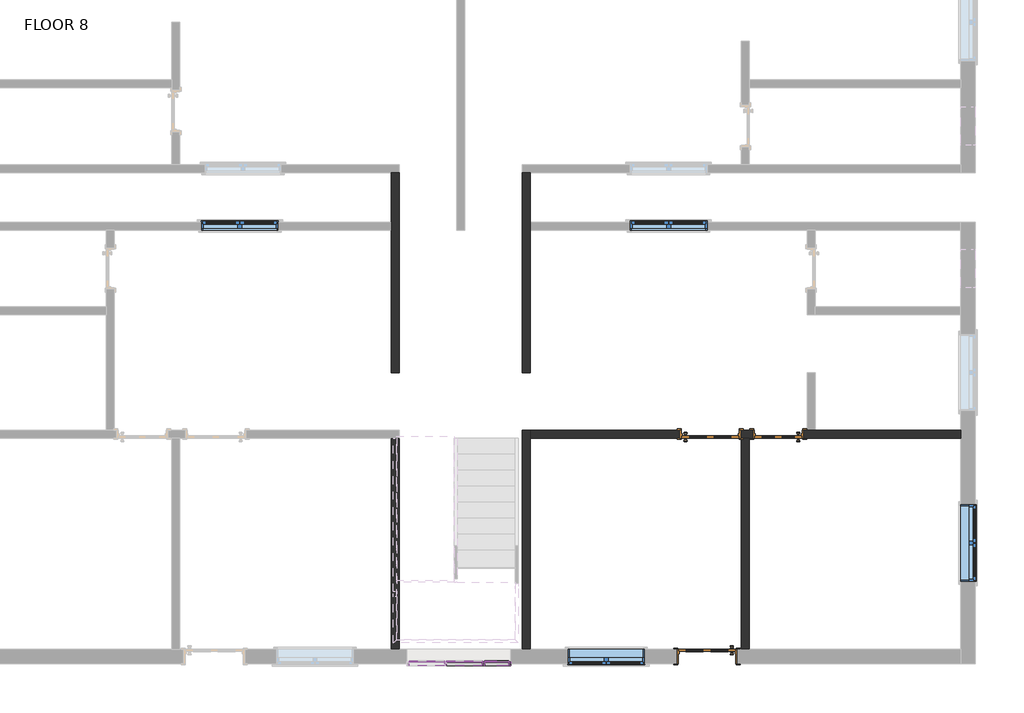
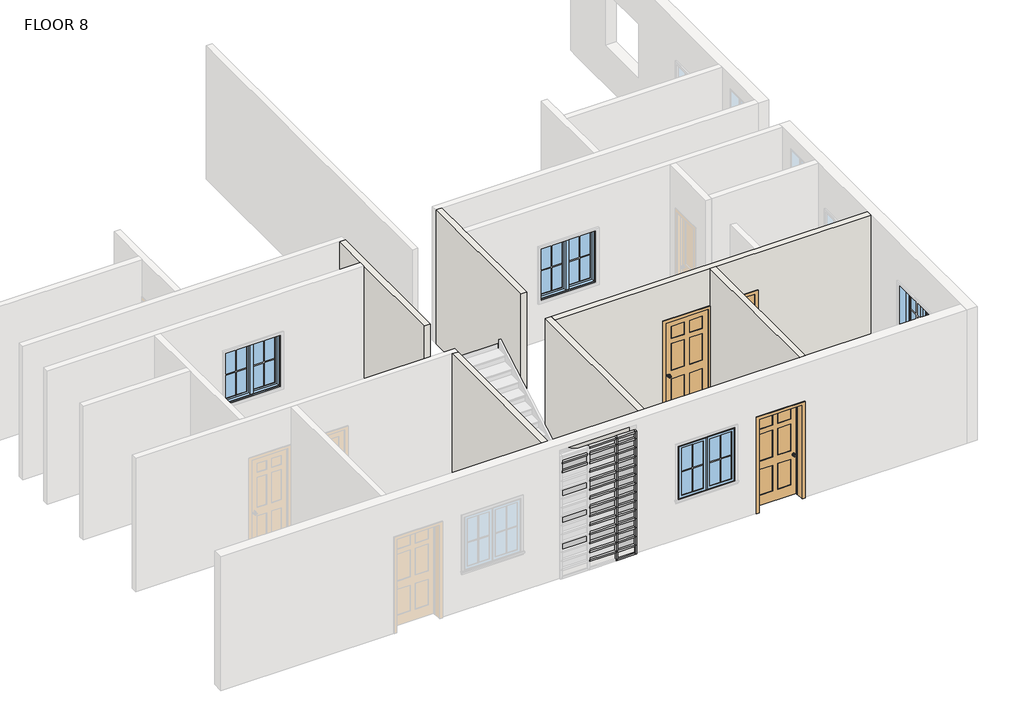
# One storey, part 2 of 4: 59 members, 22 plates, 6 walls, 4 windows, 3 doors.
"""IFC4 building model written with IfcOpenShell, lengths in millimetres."""

from ifc_helpers import new_model, si_unit, frame, origin, place, context, project, spatial, polyline, outline, extrude, faceted_brep, transform, mapped, element, save
from components import door_d66ee888, door_c610b25b, door_c5239341, member_56b223d9, member_a59c64b1, member_6a7c88b6, member_b8e7570c, member_a67f877f, member_ff422208, member_dc11c383, member_89338317, member_bd75388b, system_panel_glazed_b3845325, system_panel_glazed_23b8b45c, system_panel_glazed_a64eeae2, system_panel_glazed_c4340a26, system_panel_glazed_ac390e92, window_9200f5ac, window_c2c97eee

model = new_model("IFC4")

# Units and contexts
model_context = context("Model", 3, world=origin())
ifc_project = project(units=[si_unit("LENGTHUNIT", "METRE", prefix="MILLI")], contexts=[model_context])

# Site, building, storey
site = spatial("IfcSite", under=ifc_project)
building = spatial("IfcBuilding", under=site)
storey = spatial("IfcBuildingStorey", under=building, Name="FLOOR 8", Elevation=12744.7725604)

# Doors
placement = place(None, origin())
door_shape = door_d66ee888(model_context)
element("IfcDoor", 1, ObjectType="Door-Interior-Single-6_Panel-Wood : 30\" x 84\"", at=placement, inside=storey, context=model_context, shape_type="MappedRepresentation", body=[
    mapped(door_shape, transform((777.5862669, -4180.7343836, 12744.7725604), x_axis=(-1.0, 0.0, 0.0), y_axis=(0.0, -1.0, 0.0), z_axis=(0.0, 0.0, 1.0))),
])
door_2_shape = door_c610b25b(model_context)
element("IfcDoor", 2, ObjectType="Door-Interior-Single-6_Panel-Wood : 36\" x 84\"", at=placement, inside=storey, context=model_context, shape_type="MappedRepresentation", body=[
    mapped(door_2_shape, transform((-301.9137331, -4180.7343836, 12744.7725604), x_axis=(1.0, 0.0, 0.0), y_axis=(0.0, 1.0, 0.0), z_axis=(0.0, 0.0, 1.0))),
])
door_3_shape = door_c5239341(model_context)
element("IfcDoor", 3, ObjectType="Door-Interior-Single-6_Panel-Wood : 36\" x 84\"", at=placement, inside=storey, context=model_context, shape_type="MappedRepresentation", body=[
    mapped(door_3_shape, transform((-352.7137331, -7704.9843836, 12744.7725604), x_axis=(-1.0, 0.0, 0.0), y_axis=(0.0, -1.0, 0.0), z_axis=(0.0, 0.0, 1.0))),
])

# Members
member_shape = member_56b223d9(model_context)
element("IfcMember", 4, ObjectType="Rectangular Mullion : 1.5\" x 2.5\" rectangular", at=placement, inside=storey, context=model_context, shape_type="MappedRepresentation", body=[
    mapped(member_shape, transform((-3899.3003411, -7822.4593836, 12744.7725604), x_axis=(1.0, 0.0, 0.0), y_axis=(0.0, -1.0, 0.0), z_axis=(0.0, 0.0, -1.0))),
])
element("IfcMember", 5, ObjectType="Rectangular Mullion : 1.5\" x 2.5\" rectangular", at=placement, inside=storey, context=model_context, shape_type="MappedRepresentation", body=[
    mapped(member_shape, transform((-3899.3003411, -7822.4593836, 12947.9725604), x_axis=(1.0, 0.0, 0.0), y_axis=(0.0, -1.0, 0.0), z_axis=(0.0, 0.0, -1.0))),
])
element("IfcMember", 6, ObjectType="Rectangular Mullion : 1.5\" x 2.5\" rectangular", at=placement, inside=storey, context=model_context, shape_type="MappedRepresentation", body=[
    mapped(member_shape, transform((-3899.3003411, -7822.4593836, 13151.1725604), x_axis=(1.0, 0.0, 0.0), y_axis=(0.0, -1.0, 0.0), z_axis=(0.0, 0.0, -1.0))),
])
element("IfcMember", 7, ObjectType="Rectangular Mullion : 1.5\" x 2.5\" rectangular", at=placement, inside=storey, context=model_context, shape_type="MappedRepresentation", body=[
    mapped(member_shape, transform((-3899.3003411, -7822.4593836, 13354.3725604), x_axis=(1.0, 0.0, 0.0), y_axis=(0.0, -1.0, 0.0), z_axis=(0.0, 0.0, -1.0))),
])
element("IfcMember", 8, ObjectType="Rectangular Mullion : 1.5\" x 2.5\" rectangular", at=placement, inside=storey, context=model_context, shape_type="MappedRepresentation", body=[
    mapped(member_shape, transform((-3899.3003411, -7822.4593836, 13557.5725604), x_axis=(1.0, 0.0, 0.0), y_axis=(0.0, -1.0, 0.0), z_axis=(0.0, 0.0, -1.0))),
])
element("IfcMember", 9, ObjectType="Rectangular Mullion : 1.5\" x 2.5\" rectangular", at=placement, inside=storey, context=model_context, shape_type="MappedRepresentation", body=[
    mapped(member_shape, transform((-3899.3003411, -7822.4593836, 13760.7725604), x_axis=(1.0, 0.0, 0.0), y_axis=(0.0, -1.0, 0.0), z_axis=(0.0, 0.0, -1.0))),
])
element("IfcMember", 10, ObjectType="Rectangular Mullion : 1.5\" x 2.5\" rectangular", at=placement, inside=storey, context=model_context, shape_type="MappedRepresentation", body=[
    mapped(member_shape, transform((-3899.3003411, -7822.4593836, 13963.9725604), x_axis=(1.0, 0.0, 0.0), y_axis=(0.0, -1.0, 0.0), z_axis=(0.0, 0.0, -1.0))),
])
element("IfcMember", 11, ObjectType="Rectangular Mullion : 1.5\" x 2.5\" rectangular", at=placement, inside=storey, context=model_context, shape_type="MappedRepresentation", body=[
    mapped(member_shape, transform((-3899.3003411, -7822.4593836, 14167.1725604), x_axis=(1.0, 0.0, 0.0), y_axis=(0.0, -1.0, 0.0), z_axis=(0.0, 0.0, -1.0))),
])
element("IfcMember", 12, ObjectType="Rectangular Mullion : 1.5\" x 2.5\" rectangular", at=placement, inside=storey, context=model_context, shape_type="MappedRepresentation", body=[
    mapped(member_shape, transform((-3899.3003411, -7822.4593836, 14370.3725604), x_axis=(1.0, 0.0, 0.0), y_axis=(0.0, -1.0, 0.0), z_axis=(0.0, 0.0, -1.0))),
])
element("IfcMember", 13, ObjectType="Rectangular Mullion : 1.5\" x 2.5\" rectangular", at=placement, inside=storey, context=model_context, shape_type="MappedRepresentation", body=[
    mapped(member_shape, transform((-3899.3003411, -7822.4593836, 14573.5725604), x_axis=(1.0, 0.0, 0.0), y_axis=(0.0, -1.0, 0.0), z_axis=(0.0, 0.0, -1.0))),
])
element("IfcMember", 14, ObjectType="Rectangular Mullion : 1.5\" x 2.5\" rectangular", at=placement, inside=storey, context=model_context, shape_type="MappedRepresentation", body=[
    mapped(member_shape, transform((-3899.3003411, -7822.4593836, 14776.7725604), x_axis=(1.0, 0.0, 0.0), y_axis=(0.0, -1.0, 0.0), z_axis=(0.0, 0.0, -1.0))),
])
element("IfcMember", 15, ObjectType="Rectangular Mullion : 1.5\" x 2.5\" rectangular", at=placement, inside=storey, context=model_context, shape_type="MappedRepresentation", body=[
    mapped(member_shape, transform((-3899.3003411, -7822.4593836, 14979.9725604), x_axis=(1.0, 0.0, 0.0), y_axis=(0.0, -1.0, 0.0), z_axis=(0.0, 0.0, -1.0))),
])
element("IfcMember", 16, ObjectType="Rectangular Mullion : 1.5\" x 2.5\" rectangular", at=placement, inside=storey, context=model_context, shape_type="MappedRepresentation", body=[
    mapped(member_shape, transform((-3899.3003411, -7822.4593836, 15183.1725604), x_axis=(1.0, 0.0, 0.0), y_axis=(0.0, -1.0, 0.0), z_axis=(0.0, 0.0, -1.0))),
])
member_2_shape = member_a59c64b1(model_context)
element("IfcMember", 17, ObjectType="Rectangular Mullion : 1.5\" x 2.5\" rectangular", at=placement, inside=storey, context=model_context, shape_type="MappedRepresentation", body=[
    mapped(member_2_shape, transform((-3899.3003411, -7822.4593836, 15386.3725604), x_axis=(1.0, 0.0, 0.0), y_axis=(0.0, -1.0, 0.0), z_axis=(0.0, 0.0, -1.0))),
])
member_3_shape = member_6a7c88b6(model_context)
element("IfcMember", 18, ObjectType="Rectangular Mullion : 1.5\" x 2.5\" rectangular", at=placement, inside=storey, context=model_context, shape_type="MappedRepresentation", body=[
    mapped(member_3_shape, transform((-4527.9503411, -7822.4593836, 15183.1725604), x_axis=(0.0, 0.0, 1.0), y_axis=(0.0, -1.0, 0.0), z_axis=(1.0, 0.0, 0.0))),
])
element("IfcMember", 19, ObjectType="Rectangular Mullion : 1.5\" x 2.5\" rectangular", at=placement, inside=storey, context=model_context, shape_type="MappedRepresentation", body=[
    mapped(member_3_shape, transform((-4527.9503411, -7822.4593836, 15386.3725604), x_axis=(0.0, 0.0, 1.0), y_axis=(0.0, -1.0, 0.0), z_axis=(1.0, 0.0, 0.0))),
])
member_4_shape = member_b8e7570c(model_context)
element("IfcMember", 20, ObjectType="Rectangular Mullion : 1.5\" x 2.5\" rectangular", at=placement, inside=storey, context=model_context, shape_type="MappedRepresentation", body=[
    mapped(member_4_shape, transform((-3918.3503411, -7822.4593836, 12947.9725604), x_axis=(0.0, 0.0, 1.0), y_axis=(0.0, -1.0, 0.0), z_axis=(1.0, 0.0, 0.0))),
])
element("IfcMember", 21, ObjectType="Rectangular Mullion : 1.5\" x 2.5\" rectangular", at=placement, inside=storey, context=model_context, shape_type="MappedRepresentation", body=[
    mapped(member_4_shape, transform((-3918.3503411, -7822.4593836, 13151.1725604), x_axis=(0.0, 0.0, 1.0), y_axis=(0.0, -1.0, 0.0), z_axis=(1.0, 0.0, 0.0))),
])
element("IfcMember", 22, ObjectType="Rectangular Mullion : 1.5\" x 2.5\" rectangular", at=placement, inside=storey, context=model_context, shape_type="MappedRepresentation", body=[
    mapped(member_4_shape, transform((-3918.3503411, -7822.4593836, 13354.3725604), x_axis=(0.0, 0.0, 1.0), y_axis=(0.0, -1.0, 0.0), z_axis=(1.0, 0.0, 0.0))),
])
element("IfcMember", 23, ObjectType="Rectangular Mullion : 1.5\" x 2.5\" rectangular", at=placement, inside=storey, context=model_context, shape_type="MappedRepresentation", body=[
    mapped(member_4_shape, transform((-3918.3503411, -7822.4593836, 13557.5725604), x_axis=(0.0, 0.0, 1.0), y_axis=(0.0, -1.0, 0.0), z_axis=(1.0, 0.0, 0.0))),
])
element("IfcMember", 24, ObjectType="Rectangular Mullion : 1.5\" x 2.5\" rectangular", at=placement, inside=storey, context=model_context, shape_type="MappedRepresentation", body=[
    mapped(member_4_shape, transform((-3918.3503411, -7822.4593836, 13760.7725604), x_axis=(0.0, 0.0, 1.0), y_axis=(0.0, -1.0, 0.0), z_axis=(1.0, 0.0, 0.0))),
])
element("IfcMember", 25, ObjectType="Rectangular Mullion : 1.5\" x 2.5\" rectangular", at=placement, inside=storey, context=model_context, shape_type="MappedRepresentation", body=[
    mapped(member_4_shape, transform((-3918.3503411, -7822.4593836, 13963.9725604), x_axis=(0.0, 0.0, 1.0), y_axis=(0.0, -1.0, 0.0), z_axis=(1.0, 0.0, 0.0))),
])
element("IfcMember", 26, ObjectType="Rectangular Mullion : 1.5\" x 2.5\" rectangular", at=placement, inside=storey, context=model_context, shape_type="MappedRepresentation", body=[
    mapped(member_4_shape, transform((-3918.3503411, -7822.4593836, 14167.1725604), x_axis=(0.0, 0.0, 1.0), y_axis=(0.0, -1.0, 0.0), z_axis=(1.0, 0.0, 0.0))),
])
element("IfcMember", 27, ObjectType="Rectangular Mullion : 1.5\" x 2.5\" rectangular", at=placement, inside=storey, context=model_context, shape_type="MappedRepresentation", body=[
    mapped(member_4_shape, transform((-3918.3503411, -7822.4593836, 14370.3725604), x_axis=(0.0, 0.0, 1.0), y_axis=(0.0, -1.0, 0.0), z_axis=(1.0, 0.0, 0.0))),
])
element("IfcMember", 28, ObjectType="Rectangular Mullion : 1.5\" x 2.5\" rectangular", at=placement, inside=storey, context=model_context, shape_type="MappedRepresentation", body=[
    mapped(member_4_shape, transform((-3918.3503411, -7822.4593836, 14573.5725604), x_axis=(0.0, 0.0, 1.0), y_axis=(0.0, -1.0, 0.0), z_axis=(1.0, 0.0, 0.0))),
])
element("IfcMember", 29, ObjectType="Rectangular Mullion : 1.5\" x 2.5\" rectangular", at=placement, inside=storey, context=model_context, shape_type="MappedRepresentation", body=[
    mapped(member_4_shape, transform((-3918.3503411, -7822.4593836, 14776.7725604), x_axis=(0.0, 0.0, 1.0), y_axis=(0.0, -1.0, 0.0), z_axis=(1.0, 0.0, 0.0))),
])
element("IfcMember", 30, ObjectType="Rectangular Mullion : 1.5\" x 2.5\" rectangular", at=placement, inside=storey, context=model_context, shape_type="MappedRepresentation", body=[
    mapped(member_4_shape, transform((-3918.3503411, -7822.4593836, 14979.9725604), x_axis=(0.0, 0.0, 1.0), y_axis=(0.0, -1.0, 0.0), z_axis=(1.0, 0.0, 0.0))),
])
element("IfcMember", 31, ObjectType="Rectangular Mullion : 1.5\" x 2.5\" rectangular", at=placement, inside=storey, context=model_context, shape_type="MappedRepresentation", body=[
    mapped(member_4_shape, transform((-3918.3503411, -7822.4593836, 15183.1725604), x_axis=(0.0, 0.0, 1.0), y_axis=(0.0, -1.0, 0.0), z_axis=(1.0, 0.0, 0.0))),
])
element("IfcMember", 32, ObjectType="Rectangular Mullion : 1.5\" x 2.5\" rectangular", at=placement, inside=storey, context=model_context, shape_type="MappedRepresentation", body=[
    mapped(member_4_shape, transform((-3918.3503411, -7822.4593836, 15386.3725604), x_axis=(0.0, 0.0, 1.0), y_axis=(0.0, -1.0, 0.0), z_axis=(1.0, 0.0, 0.0))),
])
member_5_shape = member_a67f877f(model_context)
element("IfcMember", 33, ObjectType="Rectangular Mullion : 1.5\" x 2.5\" rectangular", at=placement, inside=storey, context=model_context, shape_type="MappedRepresentation", body=[
    mapped(member_5_shape, transform((-3918.3503411, -7822.4593836, 15552.1551755), x_axis=(0.0, 0.0, 1.0), y_axis=(0.0, -1.0, 0.0), z_axis=(1.0, 0.0, 0.0))),
])
member_6_shape = member_ff422208(model_context)
element("IfcMember", 34, ObjectType="Rectangular Mullion : 1.5\" x 2.5\" rectangular", at=placement, inside=storey, context=model_context, shape_type="MappedRepresentation", body=[
    mapped(member_6_shape, transform((-3466.9970483, -7822.4593836, 12744.7725604), x_axis=(1.0, 0.0, 0.0), y_axis=(0.0, -1.0, 0.0), z_axis=(0.0, 0.0, -1.0))),
])
element("IfcMember", 35, ObjectType="Rectangular Mullion : 1.5\" x 2.5\" rectangular", at=placement, inside=storey, context=model_context, shape_type="MappedRepresentation", body=[
    mapped(member_6_shape, transform((-3466.9970483, -7822.4593836, 12947.9725604), x_axis=(1.0, 0.0, 0.0), y_axis=(0.0, -1.0, 0.0), z_axis=(0.0, 0.0, -1.0))),
])
element("IfcMember", 36, ObjectType="Rectangular Mullion : 1.5\" x 2.5\" rectangular", at=placement, inside=storey, context=model_context, shape_type="MappedRepresentation", body=[
    mapped(member_6_shape, transform((-3466.9970483, -7822.4593836, 13151.1725604), x_axis=(1.0, 0.0, 0.0), y_axis=(0.0, -1.0, 0.0), z_axis=(0.0, 0.0, -1.0))),
])
element("IfcMember", 37, ObjectType="Rectangular Mullion : 1.5\" x 2.5\" rectangular", at=placement, inside=storey, context=model_context, shape_type="MappedRepresentation", body=[
    mapped(member_6_shape, transform((-3466.9970483, -7822.4593836, 13354.3725604), x_axis=(1.0, 0.0, 0.0), y_axis=(0.0, -1.0, 0.0), z_axis=(0.0, 0.0, -1.0))),
])
element("IfcMember", 38, ObjectType="Rectangular Mullion : 1.5\" x 2.5\" rectangular", at=placement, inside=storey, context=model_context, shape_type="MappedRepresentation", body=[
    mapped(member_6_shape, transform((-3466.9970483, -7822.4593836, 13557.5725604), x_axis=(1.0, 0.0, 0.0), y_axis=(0.0, -1.0, 0.0), z_axis=(0.0, 0.0, -1.0))),
])
element("IfcMember", 39, ObjectType="Rectangular Mullion : 1.5\" x 2.5\" rectangular", at=placement, inside=storey, context=model_context, shape_type="MappedRepresentation", body=[
    mapped(member_6_shape, transform((-3466.9970483, -7822.4593836, 13760.7725604), x_axis=(1.0, 0.0, 0.0), y_axis=(0.0, -1.0, 0.0), z_axis=(0.0, 0.0, -1.0))),
])
element("IfcMember", 40, ObjectType="Rectangular Mullion : 1.5\" x 2.5\" rectangular", at=placement, inside=storey, context=model_context, shape_type="MappedRepresentation", body=[
    mapped(member_6_shape, transform((-3466.9970483, -7822.4593836, 13963.9725604), x_axis=(1.0, 0.0, 0.0), y_axis=(0.0, -1.0, 0.0), z_axis=(0.0, 0.0, -1.0))),
])
element("IfcMember", 41, ObjectType="Rectangular Mullion : 1.5\" x 2.5\" rectangular", at=placement, inside=storey, context=model_context, shape_type="MappedRepresentation", body=[
    mapped(member_6_shape, transform((-3466.9970483, -7822.4593836, 14167.1725604), x_axis=(1.0, 0.0, 0.0), y_axis=(0.0, -1.0, 0.0), z_axis=(0.0, 0.0, -1.0))),
])
element("IfcMember", 42, ObjectType="Rectangular Mullion : 1.5\" x 2.5\" rectangular", at=placement, inside=storey, context=model_context, shape_type="MappedRepresentation", body=[
    mapped(member_6_shape, transform((-3466.9970483, -7822.4593836, 14370.3725604), x_axis=(1.0, 0.0, 0.0), y_axis=(0.0, -1.0, 0.0), z_axis=(0.0, 0.0, -1.0))),
])
element("IfcMember", 43, ObjectType="Rectangular Mullion : 1.5\" x 2.5\" rectangular", at=placement, inside=storey, context=model_context, shape_type="MappedRepresentation", body=[
    mapped(member_6_shape, transform((-3466.9970483, -7822.4593836, 14573.5725604), x_axis=(1.0, 0.0, 0.0), y_axis=(0.0, -1.0, 0.0), z_axis=(0.0, 0.0, -1.0))),
])
element("IfcMember", 44, ObjectType="Rectangular Mullion : 1.5\" x 2.5\" rectangular", at=placement, inside=storey, context=model_context, shape_type="MappedRepresentation", body=[
    mapped(member_6_shape, transform((-3466.9970483, -7822.4593836, 14776.7725604), x_axis=(1.0, 0.0, 0.0), y_axis=(0.0, -1.0, 0.0), z_axis=(0.0, 0.0, -1.0))),
])
element("IfcMember", 45, ObjectType="Rectangular Mullion : 1.5\" x 2.5\" rectangular", at=placement, inside=storey, context=model_context, shape_type="MappedRepresentation", body=[
    mapped(member_6_shape, transform((-3466.9970483, -7822.4593836, 14979.9725604), x_axis=(1.0, 0.0, 0.0), y_axis=(0.0, -1.0, 0.0), z_axis=(0.0, 0.0, -1.0))),
])
element("IfcMember", 46, ObjectType="Rectangular Mullion : 1.5\" x 2.5\" rectangular", at=placement, inside=storey, context=model_context, shape_type="MappedRepresentation", body=[
    mapped(member_6_shape, transform((-3466.9970483, -7822.4593836, 15183.1725604), x_axis=(1.0, 0.0, 0.0), y_axis=(0.0, -1.0, 0.0), z_axis=(0.0, 0.0, -1.0))),
])
member_7_shape = member_dc11c383(model_context)
element("IfcMember", 47, ObjectType="Rectangular Mullion : 1.5\" x 2.5\" rectangular", at=placement, inside=storey, context=model_context, shape_type="MappedRepresentation", body=[
    mapped(member_7_shape, transform((-3466.9970483, -7822.4593836, 15386.3725604), x_axis=(1.0, 0.0, 0.0), y_axis=(0.0, -1.0, 0.0), z_axis=(0.0, 0.0, -1.0))),
])
member_8_shape = member_89338317(model_context)
element("IfcMember", 48, ObjectType="Rectangular Mullion : 1.5\" x 2.5\" rectangular", at=placement, inside=storey, context=model_context, shape_type="MappedRepresentation", body=[
    mapped(member_8_shape, transform((-3505.0970483, -7822.4593836, 15552.1551755), x_axis=(0.0, 0.0, 1.0), y_axis=(0.0, -1.0, 0.0), z_axis=(1.0, 0.0, 0.0))),
])
element("IfcMember", 49, ObjectType="Rectangular Mullion : 1.5\" x 2.5\" rectangular", at=placement, inside=storey, context=model_context, shape_type="MappedRepresentation", body=[
    mapped(member_8_shape, transform((-3880.2503411, -7822.4593836, 12744.7725604), x_axis=(0.0, 0.0, -1.0), y_axis=(0.0, -1.0, 0.0), z_axis=(-1.0, 0.0, 0.0))),
])
member_9_shape = member_bd75388b(model_context)
element("IfcMember", 50, ObjectType="Rectangular Mullion : 1.5\" x 2.5\" rectangular", at=placement, inside=storey, context=model_context, shape_type="MappedRepresentation", body=[
    mapped(member_9_shape, transform((-3505.0970483, -7822.4593836, 12947.9725604), x_axis=(0.0, 0.0, 1.0), y_axis=(0.0, -1.0, 0.0), z_axis=(1.0, 0.0, 0.0))),
])
element("IfcMember", 51, ObjectType="Rectangular Mullion : 1.5\" x 2.5\" rectangular", at=placement, inside=storey, context=model_context, shape_type="MappedRepresentation", body=[
    mapped(member_9_shape, transform((-3505.0970483, -7822.4593836, 13151.1725604), x_axis=(0.0, 0.0, 1.0), y_axis=(0.0, -1.0, 0.0), z_axis=(1.0, 0.0, 0.0))),
])
element("IfcMember", 52, ObjectType="Rectangular Mullion : 1.5\" x 2.5\" rectangular", at=placement, inside=storey, context=model_context, shape_type="MappedRepresentation", body=[
    mapped(member_9_shape, transform((-3505.0970483, -7822.4593836, 13354.3725604), x_axis=(0.0, 0.0, 1.0), y_axis=(0.0, -1.0, 0.0), z_axis=(1.0, 0.0, 0.0))),
])
element("IfcMember", 53, ObjectType="Rectangular Mullion : 1.5\" x 2.5\" rectangular", at=placement, inside=storey, context=model_context, shape_type="MappedRepresentation", body=[
    mapped(member_9_shape, transform((-3505.0970483, -7822.4593836, 13557.5725604), x_axis=(0.0, 0.0, 1.0), y_axis=(0.0, -1.0, 0.0), z_axis=(1.0, 0.0, 0.0))),
])
element("IfcMember", 54, ObjectType="Rectangular Mullion : 1.5\" x 2.5\" rectangular", at=placement, inside=storey, context=model_context, shape_type="MappedRepresentation", body=[
    mapped(member_9_shape, transform((-3505.0970483, -7822.4593836, 13760.7725604), x_axis=(0.0, 0.0, 1.0), y_axis=(0.0, -1.0, 0.0), z_axis=(1.0, 0.0, 0.0))),
])
element("IfcMember", 55, ObjectType="Rectangular Mullion : 1.5\" x 2.5\" rectangular", at=placement, inside=storey, context=model_context, shape_type="MappedRepresentation", body=[
    mapped(member_9_shape, transform((-3505.0970483, -7822.4593836, 13963.9725604), x_axis=(0.0, 0.0, 1.0), y_axis=(0.0, -1.0, 0.0), z_axis=(1.0, 0.0, 0.0))),
])
element("IfcMember", 56, ObjectType="Rectangular Mullion : 1.5\" x 2.5\" rectangular", at=placement, inside=storey, context=model_context, shape_type="MappedRepresentation", body=[
    mapped(member_9_shape, transform((-3505.0970483, -7822.4593836, 14167.1725604), x_axis=(0.0, 0.0, 1.0), y_axis=(0.0, -1.0, 0.0), z_axis=(1.0, 0.0, 0.0))),
])
element("IfcMember", 57, ObjectType="Rectangular Mullion : 1.5\" x 2.5\" rectangular", at=placement, inside=storey, context=model_context, shape_type="MappedRepresentation", body=[
    mapped(member_9_shape, transform((-3505.0970483, -7822.4593836, 14370.3725604), x_axis=(0.0, 0.0, 1.0), y_axis=(0.0, -1.0, 0.0), z_axis=(1.0, 0.0, 0.0))),
])
element("IfcMember", 58, ObjectType="Rectangular Mullion : 1.5\" x 2.5\" rectangular", at=placement, inside=storey, context=model_context, shape_type="MappedRepresentation", body=[
    mapped(member_9_shape, transform((-3505.0970483, -7822.4593836, 14573.5725604), x_axis=(0.0, 0.0, 1.0), y_axis=(0.0, -1.0, 0.0), z_axis=(1.0, 0.0, 0.0))),
])
element("IfcMember", 59, ObjectType="Rectangular Mullion : 1.5\" x 2.5\" rectangular", at=placement, inside=storey, context=model_context, shape_type="MappedRepresentation", body=[
    mapped(member_9_shape, transform((-3505.0970483, -7822.4593836, 14776.7725604), x_axis=(0.0, 0.0, 1.0), y_axis=(0.0, -1.0, 0.0), z_axis=(1.0, 0.0, 0.0))),
])
element("IfcMember", 60, ObjectType="Rectangular Mullion : 1.5\" x 2.5\" rectangular", at=placement, inside=storey, context=model_context, shape_type="MappedRepresentation", body=[
    mapped(member_9_shape, transform((-3505.0970483, -7822.4593836, 14979.9725604), x_axis=(0.0, 0.0, 1.0), y_axis=(0.0, -1.0, 0.0), z_axis=(1.0, 0.0, 0.0))),
])
element("IfcMember", 61, ObjectType="Rectangular Mullion : 1.5\" x 2.5\" rectangular", at=placement, inside=storey, context=model_context, shape_type="MappedRepresentation", body=[
    mapped(member_9_shape, transform((-3505.0970483, -7822.4593836, 15183.1725604), x_axis=(0.0, 0.0, 1.0), y_axis=(0.0, -1.0, 0.0), z_axis=(1.0, 0.0, 0.0))),
])
element("IfcMember", 62, ObjectType="Rectangular Mullion : 1.5\" x 2.5\" rectangular", at=placement, inside=storey, context=model_context, shape_type="MappedRepresentation", body=[
    mapped(member_9_shape, transform((-3505.0970483, -7822.4593836, 15386.3725604), x_axis=(0.0, 0.0, 1.0), y_axis=(0.0, -1.0, 0.0), z_axis=(1.0, 0.0, 0.0))),
])

# Plates
system_panel_glazed_shape = system_panel_glazed_b3845325(model_context)
element("IfcPlate", 63, ObjectType="System Panel : Glazed", at=placement, inside=storey, context=model_context, shape_type="MappedRepresentation", body=[
    mapped(system_panel_glazed_shape, transform((-4804.1753412, -7822.4593836, 13373.4225604), x_axis=(1.0, 0.0, 0.0), y_axis=(0.0, 1.0, 0.0), z_axis=(0.0, 0.0, 1.0))),
])
element("IfcPlate", 64, ObjectType="System Panel : Glazed", at=placement, inside=storey, context=model_context, shape_type="MappedRepresentation", body=[
    mapped(system_panel_glazed_shape, transform((-4804.1753412, -7822.4593836, 13983.0225604), x_axis=(1.0, 0.0, 0.0), y_axis=(0.0, 1.0, 0.0), z_axis=(0.0, 0.0, 1.0))),
])
element("IfcPlate", 65, ObjectType="System Panel : Glazed", at=placement, inside=storey, context=model_context, shape_type="MappedRepresentation", body=[
    mapped(system_panel_glazed_shape, transform((-4804.1753412, -7822.4593836, 14592.6225604), x_axis=(1.0, 0.0, 0.0), y_axis=(0.0, 1.0, 0.0), z_axis=(0.0, 0.0, 1.0))),
])
element("IfcPlate", 66, ObjectType="System Panel : Glazed", at=placement, inside=storey, context=model_context, shape_type="MappedRepresentation", body=[
    mapped(system_panel_glazed_shape, transform((-4804.1753412, -7822.4593836, 15202.2225604), x_axis=(1.0, 0.0, 0.0), y_axis=(0.0, 1.0, 0.0), z_axis=(0.0, 0.0, 1.0))),
])
system_panel_glazed_2_shape = system_panel_glazed_23b8b45c(model_context)
element("IfcPlate", 67, ObjectType="System Panel : Glazed", at=placement, inside=storey, context=model_context, shape_type="MappedRepresentation", body=[
    mapped(system_panel_glazed_2_shape, transform((-4204.1003411, -7822.4593836, 13373.4225604), x_axis=(1.0, 0.0, 0.0), y_axis=(0.0, 1.0, 0.0), z_axis=(0.0, 0.0, 1.0))),
])
element("IfcPlate", 68, ObjectType="System Panel : Glazed", at=placement, inside=storey, context=model_context, shape_type="MappedRepresentation", body=[
    mapped(system_panel_glazed_2_shape, transform((-4204.1003411, -7822.4593836, 13983.0225604), x_axis=(1.0, 0.0, 0.0), y_axis=(0.0, 1.0, 0.0), z_axis=(0.0, 0.0, 1.0))),
])
element("IfcPlate", 69, ObjectType="System Panel : Glazed", at=placement, inside=storey, context=model_context, shape_type="MappedRepresentation", body=[
    mapped(system_panel_glazed_2_shape, transform((-4204.1003411, -7822.4593836, 14592.6225604), x_axis=(1.0, 0.0, 0.0), y_axis=(0.0, 1.0, 0.0), z_axis=(0.0, 0.0, 1.0))),
])
element("IfcPlate", 70, ObjectType="System Panel : Glazed", at=placement, inside=storey, context=model_context, shape_type="MappedRepresentation", body=[
    mapped(system_panel_glazed_2_shape, transform((-4204.1003411, -7822.4593836, 15202.2225604), x_axis=(1.0, 0.0, 0.0), y_axis=(0.0, 1.0, 0.0), z_axis=(0.0, 0.0, 1.0))),
])
system_panel_glazed_3_shape = system_panel_glazed_a64eeae2(model_context)
element("IfcPlate", 71, ObjectType="System Panel : Glazed", at=placement, inside=storey, context=model_context, shape_type="MappedRepresentation", body=[
    mapped(system_panel_glazed_3_shape, transform((-3692.6736947, -7822.4593836, 12782.8725604), x_axis=(1.0, 0.0, 0.0), y_axis=(0.0, 1.0, 0.0), z_axis=(0.0, 0.0, 1.0))),
])
system_panel_glazed_4_shape = system_panel_glazed_c4340a26(model_context)
element("IfcPlate", 72, ObjectType="System Panel : Glazed", at=placement, inside=storey, context=model_context, shape_type="MappedRepresentation", body=[
    mapped(system_panel_glazed_4_shape, transform((-3692.6736947, -7822.4593836, 12967.0225604), x_axis=(1.0, 0.0, 0.0), y_axis=(0.0, 1.0, 0.0), z_axis=(0.0, 0.0, 1.0))),
])
element("IfcPlate", 73, ObjectType="System Panel : Glazed", at=placement, inside=storey, context=model_context, shape_type="MappedRepresentation", body=[
    mapped(system_panel_glazed_4_shape, transform((-3692.6736947, -7822.4593836, 13170.2225604), x_axis=(1.0, 0.0, 0.0), y_axis=(0.0, 1.0, 0.0), z_axis=(0.0, 0.0, 1.0))),
])
element("IfcPlate", 74, ObjectType="System Panel : Glazed", at=placement, inside=storey, context=model_context, shape_type="MappedRepresentation", body=[
    mapped(system_panel_glazed_4_shape, transform((-3692.6736947, -7822.4593836, 13576.6225604), x_axis=(1.0, 0.0, 0.0), y_axis=(0.0, 1.0, 0.0), z_axis=(0.0, 0.0, 1.0))),
])
element("IfcPlate", 75, ObjectType="System Panel : Glazed", at=placement, inside=storey, context=model_context, shape_type="MappedRepresentation", body=[
    mapped(system_panel_glazed_4_shape, transform((-3692.6736947, -7822.4593836, 13779.8225604), x_axis=(1.0, 0.0, 0.0), y_axis=(0.0, 1.0, 0.0), z_axis=(0.0, 0.0, 1.0))),
])
element("IfcPlate", 76, ObjectType="System Panel : Glazed", at=placement, inside=storey, context=model_context, shape_type="MappedRepresentation", body=[
    mapped(system_panel_glazed_4_shape, transform((-3692.6736947, -7822.4593836, 14186.2225604), x_axis=(1.0, 0.0, 0.0), y_axis=(0.0, 1.0, 0.0), z_axis=(0.0, 0.0, 1.0))),
])
element("IfcPlate", 77, ObjectType="System Panel : Glazed", at=placement, inside=storey, context=model_context, shape_type="MappedRepresentation", body=[
    mapped(system_panel_glazed_4_shape, transform((-3692.6736947, -7822.4593836, 14389.4225604), x_axis=(1.0, 0.0, 0.0), y_axis=(0.0, 1.0, 0.0), z_axis=(0.0, 0.0, 1.0))),
])
element("IfcPlate", 78, ObjectType="System Panel : Glazed", at=placement, inside=storey, context=model_context, shape_type="MappedRepresentation", body=[
    mapped(system_panel_glazed_4_shape, transform((-3692.6736947, -7822.4593836, 14795.8225604), x_axis=(1.0, 0.0, 0.0), y_axis=(0.0, 1.0, 0.0), z_axis=(0.0, 0.0, 1.0))),
])
element("IfcPlate", 79, ObjectType="System Panel : Glazed", at=placement, inside=storey, context=model_context, shape_type="MappedRepresentation", body=[
    mapped(system_panel_glazed_4_shape, transform((-3692.6736947, -7822.4593836, 14999.0225604), x_axis=(1.0, 0.0, 0.0), y_axis=(0.0, 1.0, 0.0), z_axis=(0.0, 0.0, 1.0))),
])
element("IfcPlate", 80, ObjectType="System Panel : Glazed", at=placement, inside=storey, context=model_context, shape_type="MappedRepresentation", body=[
    mapped(system_panel_glazed_4_shape, transform((-3692.6736947, -7822.4593836, 13373.4225604), x_axis=(1.0, 0.0, 0.0), y_axis=(0.0, 1.0, 0.0), z_axis=(0.0, 0.0, 1.0))),
])
element("IfcPlate", 81, ObjectType="System Panel : Glazed", at=placement, inside=storey, context=model_context, shape_type="MappedRepresentation", body=[
    mapped(system_panel_glazed_4_shape, transform((-3692.6736947, -7822.4593836, 13983.0225604), x_axis=(1.0, 0.0, 0.0), y_axis=(0.0, 1.0, 0.0), z_axis=(0.0, 0.0, 1.0))),
])
element("IfcPlate", 82, ObjectType="System Panel : Glazed", at=placement, inside=storey, context=model_context, shape_type="MappedRepresentation", body=[
    mapped(system_panel_glazed_4_shape, transform((-3692.6736947, -7822.4593836, 14592.6225604), x_axis=(1.0, 0.0, 0.0), y_axis=(0.0, 1.0, 0.0), z_axis=(0.0, 0.0, 1.0))),
])
element("IfcPlate", 83, ObjectType="System Panel : Glazed", at=placement, inside=storey, context=model_context, shape_type="MappedRepresentation", body=[
    mapped(system_panel_glazed_4_shape, transform((-3692.6736947, -7822.4593836, 15202.2225604), x_axis=(1.0, 0.0, 0.0), y_axis=(0.0, 1.0, 0.0), z_axis=(0.0, 0.0, 1.0))),
])
system_panel_glazed_5_shape = system_panel_glazed_ac390e92(model_context)
element("IfcPlate", 84, ObjectType="System Panel : Glazed", at=placement, inside=storey, context=model_context, shape_type="MappedRepresentation", body=[
    mapped(system_panel_glazed_5_shape, transform((-3692.6736947, -7822.4593836, 15405.4225604), x_axis=(1.0, 0.0, 0.0), y_axis=(0.0, 1.0, 0.0), z_axis=(0.0, 0.0, 1.0))),
])

# Walls
element("IfcWall", 85, ObjectType="Inner Wall 5\"", at=placement, inside=storey, context=model_context, shape_type="Brep", body=[
    faceted_brep([(-5369.2137331, -24.6593836, 12744.7725604), (-5369.2137331, -812.0593836, 12744.7725604), (-5369.2137331, -939.0593836, 12744.7725604), (-5369.2137331, -3199.6593836, 12744.7725604), (-5369.2137331, -3199.6593836, 15792.7725604), (-5369.2137331, -939.0593836, 15792.7725604), (-5369.2137331, -812.0593836, 15792.7725604), (-5369.2137331, -24.6593836, 15792.7725604), (-5242.2137331, -24.6593836, 12744.7725604), (-5242.2137331, -24.6593836, 15792.7725604), (-5242.2137331, -3199.6593836, 15792.7725604), (-5242.2137331, -3199.6593836, 12744.7725604)], [[[0, 1, 2, 3, 4, 5, 6, 7]], [[8, 9, 10, 11]], [[3, 2, 1, 0, 8, 11]], [[4, 3, 11, 10]], [[7, 6, 5, 4, 10, 9]], [[0, 7, 9, 8]]]),
])
element("IfcWall", 86, ObjectType="Inner Wall 5\"", at=placement, inside=storey, context=model_context, shape_type="Brep", body=[
    faceted_brep([(-3286.4137331, -24.6593836, 12744.7725604), (-3286.4137331, -3199.6593836, 12744.7725604), (-3286.4137331, -3199.6593836, 15792.7725604), (-3286.4137331, -24.6593836, 15792.7725604), (-3159.4137331, -24.6593836, 12744.7725604), (-3159.4137331, -24.6593836, 15792.7725604), (-3159.4137331, -812.0593836, 15792.7725604), (-3159.4137331, -939.0593836, 15792.7725604), (-3159.4137331, -3199.6593836, 15792.7725604), (-3159.4137331, -3199.6593836, 12744.7725604), (-3159.4137331, -939.0593836, 12744.7725604), (-3159.4137331, -812.0593836, 12744.7725604)], [[[0, 1, 2, 3]], [[4, 5, 6, 7, 8, 9, 10, 11]], [[1, 0, 4, 11, 10, 9]], [[2, 1, 9, 8]], [[3, 2, 8, 7, 6, 5]], [[0, 3, 5, 4]]]),
])
element("IfcWall", 87, ObjectType="Inner Wall 5\"", at=placement, inside=storey, context=model_context, shape_type="SweptSolid", body=[
    extrude(outline(polyline([(-5242.2137331, -4241.0593836), (-5242.2137331, -7593.8593836), (-5369.2137331, -7593.8593836), (-5369.2137331, -4241.0593836), (-5242.2137331, -4241.0593836)])), frame((0.0, 0.0, 12744.7725604), z_axis=(0.0, 0.0, 1.0), x_axis=(1.0, 0.0, 0.0)), (0.0, 0.0, 1.0), 3048.0),
])
element("IfcWall", 88, ObjectType="Inner Wall 5\"", at=placement, inside=storey, context=model_context, shape_type="Brep", body=[
    faceted_brep([(-3159.4137331, -7593.8593836, 12744.7725604), (-3159.4137331, -4241.0593836, 12744.7725604), (-3159.4137331, -4114.0593836, 12744.7725604), (-3159.4137331, -4114.0593836, 15792.7725604), (-3159.4137331, -4241.0593836, 15792.7725604), (-3159.4137331, -7593.8593836, 15792.7725604), (-3286.4137331, -7593.8593836, 12744.7725604), (-3286.4137331, -7593.8593836, 15792.7725604), (-3286.4137331, -4114.0593836, 15792.7725604), (-3286.4137331, -4114.0593836, 12744.7725604)], [[[0, 1, 2, 3, 4, 5]], [[6, 7, 8, 9]], [[2, 1, 0, 6, 9]], [[5, 4, 3, 8, 7]], [[0, 5, 7, 6]], [[3, 2, 9, 8]]]),
])
element("IfcWall", 89, ObjectType="Inner Wall 5\"", at=placement, inside=storey, context=model_context, shape_type="Brep", body=[
    faceted_brep([(3673.1862669, -4241.0593836, 15792.7725604), (320.3862669, -4241.0593836, 15792.7725604), (193.3862669, -4241.0593836, 15792.7725604), (-3159.4137331, -4241.0593836, 15792.7725604), (-3159.4137331, -4241.0593836, 12744.7725604), (-784.5137331, -4241.0593836, 12744.7725604), (-784.5137331, -4241.0593836, 14903.7725604), (180.6862669, -4241.0593836, 14903.7725604), (180.6862669, -4241.0593836, 12744.7725604), (193.3862669, -4241.0593836, 12744.7725604), (320.3862669, -4241.0593836, 12744.7725604), (371.1862669, -4241.0593836, 12744.7725604), (371.1862669, -4241.0593836, 14903.7725604), (1183.9862669, -4241.0593836, 14903.7725604), (1183.9862669, -4241.0593836, 12744.7725604), (3673.1862669, -4241.0593836, 12744.7725604), (-3159.4137331, -4114.0593836, 15792.7725604), (1234.7862669, -4114.0593836, 15792.7725604), (1361.7862669, -4114.0593836, 15792.7725604), (3673.1862669, -4114.0593836, 15792.7725604), (3673.1862669, -4114.0593836, 12744.7725604), (1361.7862669, -4114.0593836, 12744.7725604), (1234.7862669, -4114.0593836, 12744.7725604), (1183.9862669, -4114.0593836, 12744.7725604), (1183.9862669, -4114.0593836, 14903.7725604), (371.1862669, -4114.0593836, 14903.7725604), (371.1862669, -4114.0593836, 12744.7725604), (180.6862669, -4114.0593836, 12744.7725604), (180.6862669, -4114.0593836, 14903.7725604), (-784.5137331, -4114.0593836, 14903.7725604), (-784.5137331, -4114.0593836, 12744.7725604), (-3159.4137331, -4114.0593836, 12744.7725604)], [[[0, 1, 2, 3, 4, 5, 6, 7, 8, 9, 10, 11, 12, 13, 14, 15]], [[16, 17, 18, 19, 20, 21, 22, 23, 24, 25, 26, 27, 28, 29, 30, 31]], [[4, 31, 30, 5]], [[20, 15, 14, 23, 22, 21]], [[8, 27, 26, 11, 10, 9]], [[3, 2, 1, 0, 19, 18, 17, 16]], [[4, 3, 16, 31]], [[0, 15, 20, 19]], [[7, 28, 27, 8]], [[28, 7, 6, 29]], [[29, 6, 5, 30]], [[25, 12, 11, 26]], [[12, 25, 24, 13]], [[13, 24, 23, 14]]]),
])
element("IfcWall", 90, ObjectType="Inner Wall 5\"", at=placement, inside=storey, context=model_context, shape_type="SweptSolid", body=[
    extrude(outline(polyline([(320.3862669, -4241.0593836), (320.3862669, -7593.8593836), (193.3862669, -7593.8593836), (193.3862669, -4241.0593836), (320.3862669, -4241.0593836)])), frame((0.0, 0.0, 12744.7725604), z_axis=(0.0, 0.0, 1.0), x_axis=(1.0, 0.0, 0.0)), (0.0, 0.0, 1.0), 3048.0),
])

# Windows
window_shape = window_9200f5ac(model_context)
element("IfcWindow", 91, ObjectType="Window-Casement-Double : 48\" x 48\"", at=placement, inside=storey, context=model_context, shape_type="MappedRepresentation", body=[
    mapped(window_shape, transform((3787.4862669, -5904.7593836, 12744.7725604), x_axis=(0.0, -1.0, 0.0), y_axis=(1.0, 0.0, 0.0), z_axis=(0.0, 0.0, 1.0))),
])
element("IfcWindow", 92, ObjectType="Window-Casement-Double : 48\" x 48\"", at=placement, inside=storey, context=model_context, shape_type="MappedRepresentation", body=[
    mapped(window_shape, transform((-1952.9137331, -7708.1593836, 12744.7725604), x_axis=(-1.0, 0.0, 0.0), y_axis=(0.0, -1.0, 0.0), z_axis=(0.0, 0.0, 1.0))),
])
window_2_shape = window_c2c97eee(model_context)
element("IfcWindow", 93, ObjectType="Window-Casement-Double : 48\" x 48\"", at=placement, inside=storey, context=model_context, shape_type="MappedRepresentation", body=[
    mapped(window_2_shape, transform((-7769.5137331, -875.5593836, 12744.7725604), x_axis=(1.0, 0.0, 0.0), y_axis=(0.0, 1.0, 0.0), z_axis=(0.0, 0.0, 1.0))),
])
element("IfcWindow", 94, ObjectType="Window-Casement-Double : 48\" x 48\"", at=placement, inside=storey, context=model_context, shape_type="MappedRepresentation", body=[
    mapped(window_2_shape, transform((-962.3137331, -875.5593836, 12744.7725604), x_axis=(1.0, 0.0, 0.0), y_axis=(0.0, 1.0, 0.0), z_axis=(0.0, 0.0, 1.0))),
])

save(model, "model.ifc")

# Revit data of these elements
# Type "Door-Interior-Single-6_Panel-Wood : 30\" x 84\""
#   Type Mark = "9"
#   Assembly Code = "C1020300"
#   Analytic Construction = "Wooden"
#   Top Rail = 0' - 4 11/16"
#   Top Panel = 0' - 8"
#   Thickness = 0' - 1 3/8"
#   Thermal Resistance (R) = 2.5876 (h·ft²·°F)/BTU
#   Swing Angle [instance default] = 90.00°
#   Stiles = 0' - 4 3/4"
#   Rough Width = 2' - 8"
#   Rough Height = 7' - 1"
#   Mullion = 0' - 4 1/2"
#   Lock Rail = 0' - 7 1/2"
#   Intermediate Rail = 0' - 4 1/2"
#   Height = 7' - 0"
#   Width = 2' - 6"
#   Heat Transfer Coefficient (U) = 0.3865 BTU/(h·ft²·°F)
#   Bottom Rail = 0' - 9 1/8"
#   Trim Material = Cherry
#   Panel Material = Cherry
#   Frame Material = Cherry
#   Door Handle Material = Aluminum
#   Visual Light Transmittance = 0
#   Solar Heat Gain Coefficient = 0
#   Wall Closure = (empty or 0)
#   Function = (empty or 0)
# Type "Door-Interior-Single-6_Panel-Wood : 36\" x 84\""
#   Type Mark = "8"
#   Assembly Code = "C1020300"
#   Analytic Construction = "Wooden"
#   Top Rail = 0' - 4 11/16"
#   Top Panel = 0' - 11"
#   Thickness = 0' - 1 3/8"
#   Thermal Resistance (R) = 2.5876 (h·ft²·°F)/BTU
#   Swing Angle [instance default] = 90.00°
#   Stiles = 0' - 4 3/4"
#   Rough Width = 3' - 2"
#   Rough Height = 7' - 1"
#   Mullion = 0' - 4 1/2"
#   Lock Rail = 0' - 7 1/2"
#   Intermediate Rail = 0' - 4 1/2"
#   Height = 7' - 0"
#   Width = 3' - 0"
#   Heat Transfer Coefficient (U) = 0.3865 BTU/(h·ft²·°F)
#   Bottom Rail = 0' - 9 1/8"
#   Trim Material = Cherry
#   Panel Material = Cherry
#   Frame Material = Cherry
#   Door Handle Material = Aluminum
#   Visual Light Transmittance = 0
#   Solar Heat Gain Coefficient = 0
#   Wall Closure = (empty or 0)
#   Function = (empty or 0)
# Type "Rectangular Mullion : 1.5\" x 2.5\" rectangular"
#   built-in parameter 1007304 = 0.208333 (stored number, unit not read)
#   built-in parameter 1007301 = 0.0625 (stored number, unit not read)
#   built-in parameter 1007300 = 0.0625 (stored number, unit not read)
# Type "System Panel : Glazed"
#   Construction Type Id = "GSP4R"
#   Analytic Construction = "1/8 in Pilkington single glazing"
#   Visual Light Transmittance = 0.9
#   Solar Heat Gain Coefficient = 0.86
#   Heat Transfer Coefficient (U) = 1.18115 BTU/(h·ft²·°F)
#   Define Thermal Properties by = 1
# Type "Inner Wall 5\""
#   Assembly Code = "B2010"
#   Layers, outside or top first: 0' - 5" "wall paint" (function 1)
# Type "Window-Casement-Double : 48\" x 48\""
#   Type Mark = "18"
#   Fire Rating = "0.5h"
#   Assembly Code = "B2020100"
#   Analytic Construction = "Double glazing - domestic"
#   Frame Extension [instance default] = 0' - 0 1/4"
#   Window Inset [instance default] = 0' - 0"
#   Wall Thickness [instance default] = 0' - 6"
#   Interior Wall Closure [instance default] = 0' - 2 1/4"
#   Half Width = 2' - 0"
#   Visual Light Transmittance = 0.81
#   Thermal Resistance (R) = 1.8146 (h·ft²·°F)/BTU
#   Solar Heat Gain Coefficient = 0.76
#   Rough Width = 4' - 0 1/2"
#   Rough Height = 4' - 0 1/2"
#   Height = 4' - 0"
#   Heat Transfer Coefficient (U) = 0.5511 BTU/(h·ft²·°F)
#   Exterior Wall Closure [instance default] = 0' - 1 1/4"
#   Extension Jamb [instance default] = 0' - 2 1/4"
#   Default Sill Height = 3' - 0"
#   Width = 4' - 0"
#   Muntin Visibility = yes
#   Interior Trim Visibility [instance default] = yes
#   Exterior Trim Visibility [instance default] = yes
#   Extension Jamb Visibility [instance default] = yes
#   Interior Trim Material = Wood - Stained
#   Muntin Pattern = Muntin Pattern_2x2 : Muntin Pattern_2x2
#   Interior Trim = Trim-Window-Interior-Flat : Picture Frame
#   Interior Frame Material = Wood - Stained
#   Glass Panel Material = Glass
#   Exterior Trim Material = Clad - White
#   Exterior Trim = Trim-Window-Exterior-Flat : with Sill
#   Exterior Frame Material = Clad - White
#   Wall Closure = (empty or 0)
# Element 1 (IfcDoor, "Door-Interior-Single-6_Panel-Wood : 30\" x 84\"")
#   Swing Angle = 90.00°
#   Phase Created = New Construction
#   Materials on its faces: "Cherry", "Aluminum"
# Elements 2, 3 (IfcDoor, "Door-Interior-Single-6_Panel-Wood : 36\" x 84\"")
#   Swing Angle = 90.00°
#   Phase Created = New Construction
#   Materials on its faces: "Cherry", "Aluminum"
# Elements 4, 5, 6, 7, 8, 9, 10, 11, 12, 13, 14, 15, 16, 17, 18, 19, 20, 21, 22, 23, 24, 25, 26, 27, 28, 29, 30, 31, 32, 33, 34, 35, 36, 37, 38, 39, 40, 41, 42, 43, 44, 45, 46, 47, 48, 49, 50, 51, 52, 53, 54, 55, 56, 57, 58, 59, 60, 61, 62 (IfcMember, "Rectangular Mullion : 1.5\" x 2.5\" rectangular")
#   Phase Created = New Construction
#   Materials on its faces: "Aluminum"
# Elements 63, 64, 65, 66, 67, 68, 69, 70, 71, 72, 73, 74, 75, 76, 77, 78, 79, 80, 81, 82, 83, 84 (IfcPlate, "System Panel : Glazed")
#   Phase Created = New Construction
#   Materials on its faces: "Glass"
# Elements 85, 86, 87, 88, 89, 90 (IfcWall, "Inner Wall 5\"")
#   Top Offset = 0' - 0"
#   Base Offset = 0' - 0"
#   Unconnected Height = 10' - 0"
#   wall height = 10' - 0"
#   Phase Created = New Construction
#   Base Constraint = FLOOR 8
#   Materials on its faces: "wall paint"
# Element 91 (IfcWindow, "Window-Casement-Double : 48\" x 48\"")
#   Mark = "171"
#   Window Inset = 0' - 0"
#   Interior Wall Closure = 0' - 2 1/4"
#   Frame Extension = 0' - 0 1/4"
#   Exterior Wall Closure = 0' - 1 1/4"
#   Interior Trim Visibility = yes
#   Exterior Trim Visibility = yes
#   Phase Created = New Construction
#   Materials on its faces: "Wood - Stained", "Glass", "Clad - White"
# Element 92 (IfcWindow, "Window-Casement-Double : 48\" x 48\"")
#   Mark = "172"
#   Window Inset = 0' - 0"
#   Interior Wall Closure = 0' - 2 1/4"
#   Frame Extension = 0' - 0 1/4"
#   Exterior Wall Closure = 0' - 1 1/4"
#   Interior Trim Visibility = yes
#   Exterior Trim Visibility = yes
#   Phase Created = New Construction
#   Materials on its faces: "Wood - Stained", "Glass", "Clad - White"
# Element 93 (IfcWindow, "Window-Casement-Double : 48\" x 48\"")
#   Mark = "176"
#   Window Inset = 0' - 0"
#   Interior Wall Closure = 0' - 2 1/4"
#   Frame Extension = 0' - 0 1/4"
#   Exterior Wall Closure = 0' - 1 1/4"
#   Interior Trim Visibility = yes
#   Exterior Trim Visibility = yes
#   Phase Created = New Construction
#   Materials on its faces: "Wood - Stained", "Glass", "Clad - White"
# Element 94 (IfcWindow, "Window-Casement-Double : 48\" x 48\"")
#   Mark = "178"
#   Window Inset = 0' - 0"
#   Interior Wall Closure = 0' - 2 1/4"
#   Frame Extension = 0' - 0 1/4"
#   Exterior Wall Closure = 0' - 1 1/4"
#   Interior Trim Visibility = yes
#   Exterior Trim Visibility = yes
#   Phase Created = New Construction
#   Materials on its faces: "Wood - Stained", "Glass", "Clad - White"
# Materials
#   "Cherry": class "Wood", colour RGB 226 177 128, transparency 0, Description = "Prunus Serotina", Cost = 0
#   "Aluminum": class "Metal", colour RGB 247 247 247, transparency 0, Description = "Aluminum 6061", Cost = 0
#   "wall paint": class "Generic", colour RGB 120 120 120, transparency 0, Cost = 0
#   "Wood - Stained": class "Wood", colour RGB 224 178 126, transparency 0, Cost = 0
#   "Glass": class "Glass", colour RGB 0 128 192, transparency 0.75, Description = "Soda Lime Glass", Cost = 0
#   "Clad - White": class "Wood", colour RGB 242 242 238, transparency 0, Cost = 0
